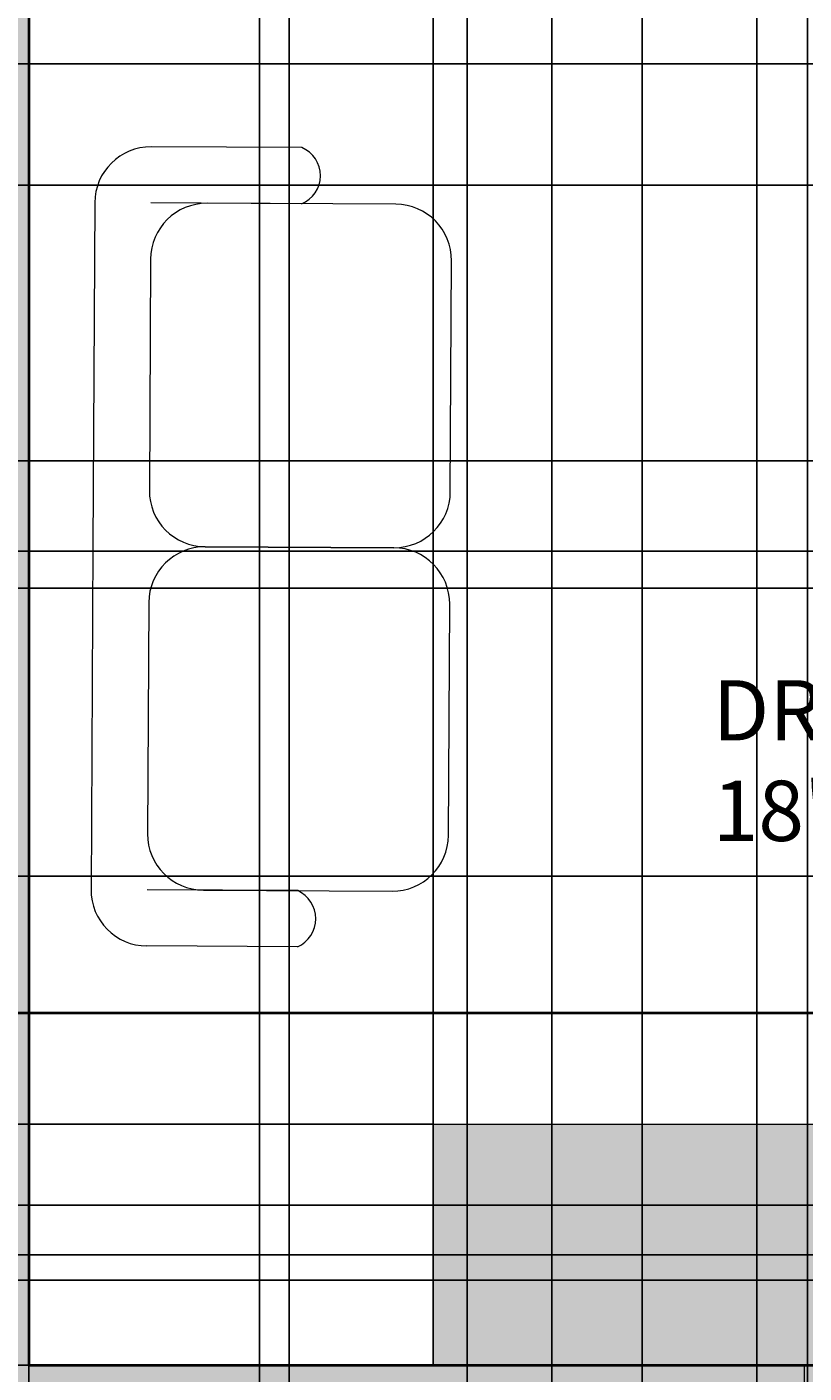
# Model space of a CAD drawing. Units: inches. Extents: x 818 to 1898, y 976 to 2364.
# Tile 23 of 96: x 1207 to 1284, y 1509 to 1643. Entities that reach past the tile are written whole.
import ezdxf

# ---------------------------------------------------------------- set-up
doc = ezdxf.new("R2010")
doc.units = ezdxf.units.IN
doc.header["$LTSCALE"] = 5
doc.header["$MEASUREMENT"] = 0
for name, color, linetype, lineweight in [('A-ANNO-DIMS', 2, 'Continuous', 18), ('A-AREA-IDEN', 7, 'Continuous', 18), ('A-FLOR-CASE', 8, 'Continuous', 18), ('A-FLOR-CASE-PATT', 33, 'Continuous', 9), ('A-FURN', 8, 'Continuous', 18), ('A-GLAZ', 4, 'Continuous', 18), ('A-WALL', 7, 'Continuous', 40)]:
    doc.layers.add(name, color=color, linetype=linetype, lineweight=lineweight)
doc.layers.add('A-GLAZ-PATT', color=141, linetype='Continuous', lineweight=9, true_color=0xadddf7)
doc.layers.add('A-WALL-PATT', color=251, linetype='Continuous', lineweight=13, true_color=0x636466)
doc.styles.get("Standard").update_dxf_attribs({"font": 'arial.ttf'})
doc.dimstyles.get("Standard").update_dxf_attribs({"dimtxt": 0.18, "dimasz": 0.18, "dimexe": 0.18, "dimexo": 0.0625, "dimgap": 0.09, "dimtad": 0, "dimtih": 1, "dimtoh": 1, "dimdec": 4, "dimzin": 0, "dimdsep": 46, "dimtxsty": 'Standard', "dimcen": 0.09, "dimadec": 0, "dimazin": 0, "dimtfac": 1, "dimtdec": 4, "dimtofl": 0, "dimtmove": 0, "dimatfit": 3, "dimfxl": 1, "dimtolj": 1, "dimtzin": 0, "dimarcsym": 0})

# ---------------------------------------------------------------- blocks, each defined once
blk = doc.blocks.new('*D59')
at = {"layer": 'A-ANNO-DIMS', "color": 0, "lineweight": -2, "ltscale": 5, "transparency": 16777216}
for p, q in [((1251.64, 2300.39), (818.03, 2300.39)), ((818.21, 2300.21), (818.21, 1669.95)), ((818.21, 1039.32), (818.21, 1669.59)), ((896.05, 1039.14), (818.03, 1039.14))]:
    blk.add_line(p, q, dxfattribs=at)
at = {"layer": 'A-ANNO-DIMS', "color": 0, "ltscale": 5, "transparency": 16777216}
for points in [[(818.18, 2300.21), (818.24, 2300.21), (818.21, 2300.39)], [(818.18, 1039.32), (818.24, 1039.32), (818.21, 1039.14)]]:
    blk.add_solid(points, dxfattribs=at)
at = {"layer": 'Defpoints', "color": 0, "ltscale": 5, "transparency": 16777216}
for p in [(818.21, 2300.39), (1251.71, 2300.39), (896.11, 1039.14)]:
    blk.add_point(p, dxfattribs=at)
at = {"layer": 'A-ANNO-DIMS', "color": 0, "ltscale": 5, "transparency": 16777216, "insert": (818.21, 1669.77), "char_height": 0.18, "attachment_point": 5}
blk.add_mtext('\\A1;1261.2', dxfattribs=at)
blk = doc.blocks.new('*D61')
at = {"layer": 'A-ANNO-DIMS', "color": 0, "lineweight": -2, "ltscale": 5, "transparency": 16777216}
for p, q in [((1071.73, 1203.03), (1071.73, 2363.87)), ((1071.91, 2363.69), (1250.94, 2363.69)), ((1430.55, 2363.69), (1251.51, 2363.69)), ((1430.73, 1203.03), (1430.73, 2363.87))]:
    blk.add_line(p, q, dxfattribs=at)
at = {"layer": 'A-ANNO-DIMS', "color": 0, "ltscale": 5, "transparency": 16777216}
for points in [[(1071.91, 2363.72), (1071.91, 2363.66), (1071.73, 2363.69)], [(1430.55, 2363.72), (1430.55, 2363.66), (1430.73, 2363.69)]]:
    blk.add_solid(points, dxfattribs=at)
at = {"layer": 'Defpoints', "color": 0, "ltscale": 5, "transparency": 16777216}
for p in [(1430.73, 2363.69), (1071.73, 1202.96), (1430.73, 1202.96)]:
    blk.add_point(p, dxfattribs=at)
at = {"layer": 'A-ANNO-DIMS', "color": 0, "ltscale": 5, "transparency": 16777216, "insert": (1251.23, 2363.69), "char_height": 0.18, "attachment_point": 5}
blk.add_mtext('\\A1;359', dxfattribs=at)
blk = doc.blocks.new('*D64')
at = {"layer": 'A-ANNO-DIMS', "color": 0, "lineweight": -2, "ltscale": 5, "transparency": 16777216}
for p, q in [((1197.73, 1501.14), (1197.73, 2363.87)), ((1197.91, 2363.69), (1313.93, 2363.69)), ((1430.55, 2363.69), (1314.52, 2363.69)), ((1430.73, 1501.14), (1430.73, 2363.87))]:
    blk.add_line(p, q, dxfattribs=at)
at = {"layer": 'A-ANNO-DIMS', "color": 0, "ltscale": 5, "transparency": 16777216}
for points in [[(1197.91, 2363.72), (1197.91, 2363.66), (1197.73, 2363.69)], [(1430.55, 2363.72), (1430.55, 2363.66), (1430.73, 2363.69)]]:
    blk.add_solid(points, dxfattribs=at)
at = {"layer": 'Defpoints', "color": 0, "ltscale": 5, "transparency": 16777216}
for p in [(1430.73, 2363.69), (1197.73, 1501.08), (1430.73, 1501.08)]:
    blk.add_point(p, dxfattribs=at)
at = {"layer": 'A-ANNO-DIMS', "color": 0, "ltscale": 5, "transparency": 16777216, "insert": (1314.23, 2363.69), "char_height": 0.18, "attachment_point": 5}
blk.add_mtext('\\A1;233', dxfattribs=at)
blk = doc.blocks.new('*D95')
at = {"layer": 'A-ANNO-DIMS', "color": 0, "lineweight": -2, "ltscale": 5, "transparency": 16777216}
for p, q in [((1173.54, 1071.12), (1173.54, 2363.87)), ((1173.72, 2363.69), (1201.29, 2363.69)), ((1229.47, 2363.69), (1201.9, 2363.69)), ((1229.65, 1071.12), (1229.65, 2363.87))]:
    blk.add_line(p, q, dxfattribs=at)
at = {"layer": 'A-ANNO-DIMS', "color": 0, "ltscale": 5, "transparency": 16777216}
for points in [[(1173.72, 2363.72), (1173.72, 2363.66), (1173.54, 2363.69)], [(1229.47, 2363.72), (1229.47, 2363.66), (1229.65, 2363.69)]]:
    blk.add_solid(points, dxfattribs=at)
at = {"layer": 'Defpoints', "color": 0, "ltscale": 5, "transparency": 16777216}
for p in [(1229.65, 2363.69), (1173.54, 1071.06), (1229.65, 1071.06)]:
    blk.add_point(p, dxfattribs=at)
at = {"layer": 'A-ANNO-DIMS', "color": 0, "ltscale": 5, "transparency": 16777216, "insert": (1201.59, 2363.69), "char_height": 0.18, "attachment_point": 5}
blk.add_mtext('\\A1;56.1', dxfattribs=at)
blk = doc.blocks.new('*D96')
at = {"layer": 'A-ANNO-DIMS', "color": 0, "lineweight": -2, "ltscale": 5, "transparency": 16777216}
for p, q in [((1229.65, 1071.12), (1229.65, 2363.87)), ((1229.83, 2363.69), (1256.52, 2363.69)), ((1283.99, 2363.69), (1257.3, 2363.69)), ((1284.17, 1071.12), (1284.17, 2363.87))]:
    blk.add_line(p, q, dxfattribs=at)
at = {"layer": 'A-ANNO-DIMS', "color": 0, "ltscale": 5, "transparency": 16777216}
for points in [[(1229.83, 2363.72), (1229.83, 2363.66), (1229.65, 2363.69)], [(1283.99, 2363.72), (1283.99, 2363.66), (1284.17, 2363.69)]]:
    blk.add_solid(points, dxfattribs=at)
at = {"layer": 'Defpoints', "color": 0, "ltscale": 5, "transparency": 16777216}
for p in [(1284.17, 2363.69), (1229.65, 1071.06), (1284.17, 1071.06)]:
    blk.add_point(p, dxfattribs=at)
at = {"layer": 'A-ANNO-DIMS', "color": 0, "ltscale": 5, "transparency": 16777216, "insert": (1256.91, 2363.69), "char_height": 0.18, "attachment_point": 5}
blk.add_mtext('\\A1;54.52', dxfattribs=at)
blk = doc.blocks.new('*D117')
at = {"layer": 'A-ANNO-DIMS', "color": 0, "lineweight": -2, "ltscale": 5, "transparency": 16777216}
for p, q in [((1766.29, 1545.18), (818.03, 1545.18)), ((818.21, 1545), (818.21, 1501.18)), ((818.21, 1456.99), (818.21, 1500.81)), ((1766.29, 1456.81), (818.03, 1456.81))]:
    blk.add_line(p, q, dxfattribs=at)
at = {"layer": 'A-ANNO-DIMS', "color": 0, "ltscale": 5, "transparency": 16777216}
for points in [[(818.18, 1545), (818.24, 1545), (818.21, 1545.18)], [(818.18, 1456.99), (818.24, 1456.99), (818.21, 1456.81)]]:
    blk.add_solid(points, dxfattribs=at)
at = {"layer": 'Defpoints', "color": 0, "ltscale": 5, "transparency": 16777216}
for p in [(818.21, 1545.18), (1766.35, 1545.18), (1766.35, 1456.81)]:
    blk.add_point(p, dxfattribs=at)
at = {"layer": 'A-ANNO-DIMS', "color": 0, "ltscale": 5, "transparency": 16777216, "insert": (818.21, 1501), "char_height": 0.18, "attachment_point": 5}
blk.add_mtext('\\A1;88.37', dxfattribs=at)
blk = doc.blocks.new('*D118')
at = {"layer": 'A-ANNO-DIMS', "color": 0, "lineweight": -2, "ltscale": 5, "transparency": 16777216}
for p, q in [((1766.29, 1627.51), (818.03, 1627.51)), ((818.21, 1627.33), (818.21, 1586.53)), ((818.21, 1545.36), (818.21, 1586.16)), ((1766.29, 1545.18), (818.03, 1545.18))]:
    blk.add_line(p, q, dxfattribs=at)
at = {"layer": 'A-ANNO-DIMS', "color": 0, "ltscale": 5, "transparency": 16777216}
for points in [[(818.18, 1627.33), (818.24, 1627.33), (818.21, 1627.51)], [(818.18, 1545.36), (818.24, 1545.36), (818.21, 1545.18)]]:
    blk.add_solid(points, dxfattribs=at)
at = {"layer": 'Defpoints', "color": 0, "ltscale": 5, "transparency": 16777216}
for p in [(818.21, 1627.51), (1766.35, 1627.51), (1766.35, 1545.18)]:
    blk.add_point(p, dxfattribs=at)
at = {"layer": 'A-ANNO-DIMS', "color": 0, "ltscale": 5, "transparency": 16777216, "insert": (818.21, 1586.34), "char_height": 0.18, "attachment_point": 5}
blk.add_mtext('\\A1;82.32', dxfattribs=at)
blk = doc.blocks.new('*D119')
at = {"layer": 'A-ANNO-DIMS', "color": 0, "lineweight": -2, "ltscale": 5, "transparency": 16777216}
for p, q in [((1766.29, 1716.99), (818.03, 1716.99)), ((818.21, 1716.81), (818.21, 1672.43)), ((818.21, 1627.69), (818.21, 1672.06)), ((1766.29, 1627.51), (818.03, 1627.51))]:
    blk.add_line(p, q, dxfattribs=at)
at = {"layer": 'A-ANNO-DIMS', "color": 0, "ltscale": 5, "transparency": 16777216}
for points in [[(818.18, 1716.81), (818.24, 1716.81), (818.21, 1716.99)], [(818.18, 1627.69), (818.24, 1627.69), (818.21, 1627.51)]]:
    blk.add_solid(points, dxfattribs=at)
at = {"layer": 'Defpoints', "color": 0, "ltscale": 5, "transparency": 16777216}
for p in [(818.21, 1716.99), (1766.35, 1716.99), (1766.35, 1627.51)]:
    blk.add_point(p, dxfattribs=at)
at = {"layer": 'A-ANNO-DIMS', "color": 0, "ltscale": 5, "transparency": 16777216, "insert": (818.21, 1672.25), "char_height": 0.18, "attachment_point": 5}
blk.add_mtext('\\A1;89.48', dxfattribs=at)
blk = doc.blocks.new('*D145')
at = {"layer": 'A-ANNO-DIMS', "color": 0, "lineweight": -2, "ltscale": 5, "transparency": 16777216}
for p, q in [((1197.39, 2122.31), (1197.39, 975.66)), ((1232.61, 2122.31), (1232.61, 975.66)), ((1197.57, 975.84), (1214.61, 975.84)), ((1232.43, 975.84), (1215.39, 975.84))]:
    blk.add_line(p, q, dxfattribs=at)
at = {"layer": 'A-ANNO-DIMS', "color": 0, "ltscale": 5, "transparency": 16777216}
for points in [[(1197.57, 975.87), (1197.57, 975.81), (1197.39, 975.84)], [(1232.43, 975.87), (1232.43, 975.81), (1232.61, 975.84)]]:
    blk.add_solid(points, dxfattribs=at)
at = {"layer": 'Defpoints', "color": 0, "ltscale": 5, "transparency": 16777216}
for p in [(1197.39, 2122.38), (1232.61, 2122.38), (1232.61, 975.84)]:
    blk.add_point(p, dxfattribs=at)
at = {"layer": 'A-ANNO-DIMS', "color": 0, "ltscale": 5, "transparency": 16777216, "insert": (1215, 975.84), "char_height": 0.18, "attachment_point": 5}
blk.add_mtext('\\A1;35.22', dxfattribs=at)
blk = doc.blocks.new('*D159')
at = {"layer": 'A-ANNO-DIMS', "color": 0, "lineweight": -2, "ltscale": 5, "transparency": 16777216}
for p, q in [((1206.73, 1687.02), (1206.73, 975.66)), ((1463.73, 1687.02), (1463.73, 975.66)), ((1206.91, 975.84), (1334.93, 975.84)), ((1463.55, 975.84), (1335.52, 975.84))]:
    blk.add_line(p, q, dxfattribs=at)
at = {"layer": 'A-ANNO-DIMS', "color": 0, "ltscale": 5, "transparency": 16777216}
for points in [[(1206.91, 975.87), (1206.91, 975.81), (1206.73, 975.84)], [(1463.55, 975.87), (1463.55, 975.81), (1463.73, 975.84)]]:
    blk.add_solid(points, dxfattribs=at)
at = {"layer": 'Defpoints', "color": 0, "ltscale": 5, "transparency": 16777216}
for p in [(1206.73, 1687.08), (1463.73, 1687.08), (1463.73, 975.84)]:
    blk.add_point(p, dxfattribs=at)
at = {"layer": 'A-ANNO-DIMS', "color": 0, "ltscale": 5, "transparency": 16777216, "insert": (1335.23, 975.84), "char_height": 0.18, "attachment_point": 5}
blk.add_mtext('\\A1;257', dxfattribs=at)
blk = doc.blocks.new('*D181')
at = {"layer": 'A-ANNO-DIMS', "color": 0, "lineweight": -2, "ltscale": 5, "transparency": 16777216}
for p, q in [((1599.66, 1639.58), (818.03, 1639.58)), ((818.21, 1639.4), (818.21, 1620.01)), ((818.21, 1600.26), (818.21, 1619.65)), ((1619.66, 1600.08), (818.03, 1600.08))]:
    blk.add_line(p, q, dxfattribs=at)
at = {"layer": 'A-ANNO-DIMS', "color": 0, "ltscale": 5, "transparency": 16777216}
for points in [[(818.18, 1639.4), (818.24, 1639.4), (818.21, 1639.58)], [(818.18, 1600.26), (818.24, 1600.26), (818.21, 1600.08)]]:
    blk.add_solid(points, dxfattribs=at)
at = {"layer": 'Defpoints', "color": 0, "ltscale": 5, "transparency": 16777216}
for p in [(1599.73, 1639.58), (818.21, 1600.08), (1619.73, 1600.08)]:
    blk.add_point(p, dxfattribs=at)
at = {"layer": 'A-ANNO-DIMS', "color": 0, "ltscale": 5, "transparency": 16777216, "insert": (818.21, 1619.83), "char_height": 0.18, "attachment_point": 5}
blk.add_mtext('\\A1;39.5', dxfattribs=at)
blk = doc.blocks.new('*D187')
at = {"layer": 'A-ANNO-DIMS', "color": 0, "lineweight": -2, "ltscale": 5, "transparency": 16777216}
for p, q in [((1705.66, 1545.08), (818.03, 1545.08)), ((818.21, 1544.9), (818.21, 1533.26)), ((818.21, 1521.26), (818.21, 1532.9)), ((1705.66, 1521.08), (818.03, 1521.08))]:
    blk.add_line(p, q, dxfattribs=at)
at = {"layer": 'A-ANNO-DIMS', "color": 0, "ltscale": 5, "transparency": 16777216}
for points in [[(818.18, 1544.9), (818.24, 1544.9), (818.21, 1545.08)], [(818.18, 1521.26), (818.24, 1521.26), (818.21, 1521.08)]]:
    blk.add_solid(points, dxfattribs=at)
at = {"layer": 'Defpoints', "color": 0, "ltscale": 5, "transparency": 16777216}
for p in [(818.21, 1545.08), (1705.73, 1545.08), (1705.73, 1521.08)]:
    blk.add_point(p, dxfattribs=at)
at = {"layer": 'A-ANNO-DIMS', "color": 0, "ltscale": 5, "transparency": 16777216, "insert": (818.21, 1533.08), "char_height": 0.18, "attachment_point": 5}
blk.add_mtext('\\A1;24', dxfattribs=at)
blk = doc.blocks.new('*D194')
at = {"layer": 'A-ANNO-DIMS', "color": 0, "lineweight": -2, "ltscale": 5, "transparency": 16777216}
for p, q in [((1616.66, 1591.08), (818.03, 1591.08)), ((818.21, 1590.9), (818.21, 1575.1)), ((818.21, 1558.93), (818.21, 1574.73)), ((1616.66, 1558.75), (818.03, 1558.75))]:
    blk.add_line(p, q, dxfattribs=at)
at = {"layer": 'A-ANNO-DIMS', "color": 0, "ltscale": 5, "transparency": 16777216}
for points in [[(818.18, 1590.9), (818.24, 1590.9), (818.21, 1591.08)], [(818.18, 1558.93), (818.24, 1558.93), (818.21, 1558.75)]]:
    blk.add_solid(points, dxfattribs=at)
at = {"layer": 'Defpoints', "color": 0, "ltscale": 5, "transparency": 16777216}
for p in [(818.21, 1591.08), (1616.73, 1591.08), (1616.73, 1558.75)]:
    blk.add_point(p, dxfattribs=at)
at = {"layer": 'A-ANNO-DIMS', "color": 0, "ltscale": 5, "transparency": 16777216, "insert": (818.21, 1574.92), "char_height": 0.18, "attachment_point": 5}
blk.add_mtext('\\A1;32.326', dxfattribs=at)
blk = doc.blocks.new('*D201')
at = {"layer": 'A-ANNO-DIMS', "color": 0, "lineweight": -2, "ltscale": 5, "transparency": 16777216}
for p, q in [((1678.27, 1518.56), (818.03, 1518.56)), ((818.21, 1518.38), (818.21, 1498.18)), ((818.21, 1477.61), (818.21, 1497.81)), ((1678.27, 1477.43), (818.03, 1477.43))]:
    blk.add_line(p, q, dxfattribs=at)
at = {"layer": 'A-ANNO-DIMS', "color": 0, "ltscale": 5, "transparency": 16777216}
for points in [[(818.18, 1518.38), (818.24, 1518.38), (818.21, 1518.56)], [(818.18, 1477.61), (818.24, 1477.61), (818.21, 1477.43)]]:
    blk.add_solid(points, dxfattribs=at)
at = {"layer": 'Defpoints', "color": 0, "ltscale": 5, "transparency": 16777216}
for p in [(818.21, 1518.56), (1678.33, 1518.56), (1678.33, 1477.43)]:
    blk.add_point(p, dxfattribs=at)
at = {"layer": 'A-ANNO-DIMS', "color": 0, "ltscale": 5, "transparency": 16777216, "insert": (818.21, 1497.99), "char_height": 0.18, "attachment_point": 5}
blk.add_mtext('\\A1;41.135', dxfattribs=at)
blk = doc.blocks.new('*D233')
at = {"layer": 'A-ANNO-DIMS', "color": 0, "lineweight": -2, "ltscale": 5, "transparency": 16777216}
for p, q in [((1267.73, 2044.02), (1267.73, 975.66)), ((1303.93, 2008.33), (1303.93, 975.66)), ((1267.91, 975.84), (1285.36, 975.84)), ((1303.75, 975.84), (1286.29, 975.84))]:
    blk.add_line(p, q, dxfattribs=at)
at = {"layer": 'A-ANNO-DIMS', "color": 0, "ltscale": 5, "transparency": 16777216}
for points in [[(1267.91, 975.87), (1267.91, 975.81), (1267.73, 975.84)], [(1303.75, 975.87), (1303.75, 975.81), (1303.93, 975.84)]]:
    blk.add_solid(points, dxfattribs=at)
at = {"layer": 'Defpoints', "color": 0, "ltscale": 5, "transparency": 16777216}
for p in [(1267.73, 2044.08), (1303.93, 2008.39), (1303.93, 975.84)]:
    blk.add_point(p, dxfattribs=at)
at = {"layer": 'A-ANNO-DIMS', "color": 0, "ltscale": 5, "transparency": 16777216, "insert": (1285.83, 975.84), "char_height": 0.18, "attachment_point": 5}
blk.add_mtext('\\A1;36.206', dxfattribs=at)
blk = doc.blocks.new('*D251')
at = {"layer": 'A-ANNO-DIMS', "color": 0, "lineweight": -2, "ltscale": 5, "transparency": 16777216}
for p, q in [((1250.3, 1878.33), (1250.3, 975.66)), ((1258.73, 1878.33), (1258.73, 975.66)), ((1250.48, 975.84), (1254.12, 975.84)), ((1258.55, 975.84), (1254.91, 975.84))]:
    blk.add_line(p, q, dxfattribs=at)
at = {"layer": 'A-ANNO-DIMS', "color": 0, "ltscale": 5, "transparency": 16777216}
for points in [[(1250.48, 975.87), (1250.48, 975.81), (1250.3, 975.84)], [(1258.55, 975.87), (1258.55, 975.81), (1258.73, 975.84)]]:
    blk.add_solid(points, dxfattribs=at)
at = {"layer": 'Defpoints', "color": 0, "ltscale": 5, "transparency": 16777216}
for p in [(1250.3, 1878.39), (1258.73, 1878.39), (1258.73, 975.84)]:
    blk.add_point(p, dxfattribs=at)
at = {"layer": 'A-ANNO-DIMS', "color": 0, "ltscale": 5, "transparency": 16777216, "insert": (1254.51, 975.84), "char_height": 0.18, "attachment_point": 5}
blk.add_mtext('\\A1;8.422', dxfattribs=at)
blk = doc.blocks.new('*D254')
at = {"layer": 'A-ANNO-DIMS', "color": 0, "lineweight": -2, "ltscale": 5, "transparency": 16777216}
for p, q in [((1267.73, 2044.02), (1267.73, 975.66)), ((1330.3, 2044.02), (1330.3, 975.66)), ((1267.91, 975.84), (1298.62, 975.84)), ((1330.12, 975.84), (1299.41, 975.84))]:
    blk.add_line(p, q, dxfattribs=at)
at = {"layer": 'A-ANNO-DIMS', "color": 0, "ltscale": 5, "transparency": 16777216}
for points in [[(1267.91, 975.87), (1267.91, 975.81), (1267.73, 975.84)], [(1330.12, 975.87), (1330.12, 975.81), (1330.3, 975.84)]]:
    blk.add_solid(points, dxfattribs=at)
at = {"layer": 'Defpoints', "color": 0, "ltscale": 5, "transparency": 16777216}
for p in [(1267.73, 2044.08), (1330.3, 2044.08), (1330.3, 975.84)]:
    blk.add_point(p, dxfattribs=at)
at = {"layer": 'A-ANNO-DIMS', "color": 0, "ltscale": 5, "transparency": 16777216, "insert": (1299.02, 975.84), "char_height": 0.18, "attachment_point": 5}
blk.add_mtext('\\A1;62.58', dxfattribs=at)
blk = doc.blocks.new('*D269')
at = {"layer": 'A-ANNO-DIMS', "color": 0, "lineweight": -2, "ltscale": 5, "transparency": 16777216}
for p, q in [((1246.94, 1534.14), (1246.94, 2363.87)), ((1247.12, 2363.69), (1293.71, 2363.69)), ((1341.08, 2363.69), (1294.49, 2363.69)), ((1341.26, 1534.14), (1341.26, 2363.87))]:
    blk.add_line(p, q, dxfattribs=at)
at = {"layer": 'A-ANNO-DIMS', "color": 0, "ltscale": 5, "transparency": 16777216}
for points in [[(1247.12, 2363.72), (1247.12, 2363.66), (1246.94, 2363.69)], [(1341.08, 2363.72), (1341.08, 2363.66), (1341.26, 2363.69)]]:
    blk.add_solid(points, dxfattribs=at)
at = {"layer": 'Defpoints', "color": 0, "ltscale": 5, "transparency": 16777216}
for p in [(1341.26, 2363.69), (1246.94, 1534.08), (1341.26, 1534.08)]:
    blk.add_point(p, dxfattribs=at)
at = {"layer": 'A-ANNO-DIMS', "color": 0, "ltscale": 5, "transparency": 16777216, "insert": (1294.1, 2363.69), "char_height": 0.18, "attachment_point": 5}
blk.add_mtext('\\A1;94.32', dxfattribs=at)
blk = doc.blocks.new('*D270')
at = {"layer": 'A-ANNO-DIMS', "color": 0, "lineweight": -2, "ltscale": 5, "transparency": 16777216}
for p, q in [((1246.88, 1534.08), (818.03, 1534.08)), ((818.21, 1533.9), (818.21, 1522.26)), ((818.21, 1510.26), (818.21, 1521.9)), ((1246.88, 1510.08), (818.03, 1510.08))]:
    blk.add_line(p, q, dxfattribs=at)
at = {"layer": 'A-ANNO-DIMS', "color": 0, "ltscale": 5, "transparency": 16777216}
for points in [[(818.18, 1533.9), (818.24, 1533.9), (818.21, 1534.08)], [(818.18, 1510.26), (818.24, 1510.26), (818.21, 1510.08)]]:
    blk.add_solid(points, dxfattribs=at)
at = {"layer": 'Defpoints', "color": 0, "ltscale": 5, "transparency": 16777216}
for p in [(818.21, 1534.08), (1246.94, 1534.08), (1246.94, 1510.08)]:
    blk.add_point(p, dxfattribs=at)
at = {"layer": 'A-ANNO-DIMS', "color": 0, "ltscale": 5, "transparency": 16777216, "insert": (818.21, 1522.08), "char_height": 0.18, "attachment_point": 5}
blk.add_mtext('\\A1;24', dxfattribs=at)
blk = doc.blocks.new('*D271')
at = {"layer": 'A-ANNO-DIMS', "color": 0, "lineweight": -2, "ltscale": 5, "transparency": 16777216}
for p, q in [((1206.73, 1510.14), (1206.73, 2363.87)), ((1206.91, 2363.69), (1226.45, 2363.69)), ((1246.76, 2363.69), (1227.21, 2363.69)), ((1246.94, 1510.14), (1246.94, 2363.87))]:
    blk.add_line(p, q, dxfattribs=at)
at = {"layer": 'A-ANNO-DIMS', "color": 0, "ltscale": 5, "transparency": 16777216}
for points in [[(1206.91, 2363.72), (1206.91, 2363.66), (1206.73, 2363.69)], [(1246.76, 2363.72), (1246.76, 2363.66), (1246.94, 2363.69)]]:
    blk.add_solid(points, dxfattribs=at)
at = {"layer": 'Defpoints', "color": 0, "ltscale": 5, "transparency": 16777216}
for p in [(1246.94, 2363.69), (1206.73, 1510.08), (1246.94, 1510.08)]:
    blk.add_point(p, dxfattribs=at)
at = {"layer": 'A-ANNO-DIMS', "color": 0, "ltscale": 5, "transparency": 16777216, "insert": (1226.83, 2363.69), "char_height": 0.18, "attachment_point": 5}
blk.add_mtext('\\A1;40.21', dxfattribs=at)
blk = doc.blocks.new('*D272')
at = {"layer": 'A-ANNO-DIMS', "color": 0, "lineweight": -2, "ltscale": 5, "transparency": 16777216}
for p, q in [((1406.66, 1587.42), (818.03, 1587.42)), ((818.21, 1587.24), (818.21, 1556.89)), ((818.21, 1526.18), (818.21, 1556.52)), ((1406.66, 1526), (818.03, 1526))]:
    blk.add_line(p, q, dxfattribs=at)
at = {"layer": 'A-ANNO-DIMS', "color": 0, "ltscale": 5, "transparency": 16777216}
for points in [[(818.18, 1587.24), (818.24, 1587.24), (818.21, 1587.42)], [(818.18, 1526.18), (818.24, 1526.18), (818.21, 1526)]]:
    blk.add_solid(points, dxfattribs=at)
at = {"layer": 'Defpoints', "color": 0, "ltscale": 5, "transparency": 16777216}
for p in [(818.21, 1587.42), (1406.73, 1587.42), (1406.73, 1526)]:
    blk.add_point(p, dxfattribs=at)
at = {"layer": 'A-ANNO-DIMS', "color": 0, "ltscale": 5, "transparency": 16777216, "insert": (818.21, 1556.71), "char_height": 0.18, "attachment_point": 5}
blk.add_mtext('\\A1;61.42', dxfattribs=at)
blk = doc.blocks.new('*D278')
at = {"layer": 'A-ANNO-DIMS', "color": 0, "lineweight": -2, "ltscale": 5, "transparency": 16777216}
for p, q in [((1324.03, 1700.74), (1324.03, 975.66)), ((1267.73, 1696.02), (1267.73, 975.66)), ((1267.91, 975.84), (1295.5, 975.84)), ((1323.85, 975.84), (1296.26, 975.84))]:
    blk.add_line(p, q, dxfattribs=at)
at = {"layer": 'A-ANNO-DIMS', "color": 0, "ltscale": 5, "transparency": 16777216}
for points in [[(1267.91, 975.87), (1267.91, 975.81), (1267.73, 975.84)], [(1323.85, 975.87), (1323.85, 975.81), (1324.03, 975.84)]]:
    blk.add_solid(points, dxfattribs=at)
at = {"layer": 'Defpoints', "color": 0, "ltscale": 5, "transparency": 16777216}
for p in [(1324.03, 1700.81), (1267.73, 1696.08), (1324.03, 975.84)]:
    blk.add_point(p, dxfattribs=at)
at = {"layer": 'A-ANNO-DIMS', "color": 0, "ltscale": 5, "transparency": 16777216, "insert": (1295.88, 975.84), "char_height": 0.18, "attachment_point": 5}
blk.add_mtext('\\A1;56.31', dxfattribs=at)
blk = doc.blocks.new('*D279')
at = {"layer": 'A-ANNO-DIMS', "color": 0, "lineweight": -2, "ltscale": 5, "transparency": 16777216}
for p, q in [((1279.13, 1713.75), (1279.13, 975.66)), ((1267.73, 1696.02), (1267.73, 975.66)), ((1267.91, 975.84), (1273.11, 975.84)), ((1278.95, 975.84), (1273.74, 975.84))]:
    blk.add_line(p, q, dxfattribs=at)
at = {"layer": 'A-ANNO-DIMS', "color": 0, "ltscale": 5, "transparency": 16777216}
for points in [[(1267.91, 975.87), (1267.91, 975.81), (1267.73, 975.84)], [(1278.95, 975.87), (1278.95, 975.81), (1279.13, 975.84)]]:
    blk.add_solid(points, dxfattribs=at)
at = {"layer": 'Defpoints', "color": 0, "ltscale": 5, "transparency": 16777216}
for p in [(1279.13, 1713.82), (1267.73, 1696.08), (1267.73, 975.84)]:
    blk.add_point(p, dxfattribs=at)
at = {"layer": 'A-ANNO-DIMS', "color": 0, "ltscale": 5, "transparency": 16777216, "insert": (1273.43, 975.84), "char_height": 0.18, "attachment_point": 5}
blk.add_mtext('\\A1;11.4', dxfattribs=at)
blk = doc.blocks.new('*D283')
at = {"layer": 'A-ANNO-DIMS', "color": 0, "lineweight": -2, "ltscale": 5, "transparency": 16777216}
for p, q in [((1351.6, 1761.39), (1351.6, 975.66)), ((1267.73, 1696.02), (1267.73, 975.66)), ((1267.91, 975.84), (1309.27, 975.84)), ((1351.42, 975.84), (1310.06, 975.84))]:
    blk.add_line(p, q, dxfattribs=at)
at = {"layer": 'A-ANNO-DIMS', "color": 0, "ltscale": 5, "transparency": 16777216}
for points in [[(1267.91, 975.87), (1267.91, 975.81), (1267.73, 975.84)], [(1351.42, 975.87), (1351.42, 975.81), (1351.6, 975.84)]]:
    blk.add_solid(points, dxfattribs=at)
at = {"layer": 'Defpoints', "color": 0, "ltscale": 5, "transparency": 16777216}
for p in [(1351.6, 1761.45), (1267.73, 1696.08), (1351.6, 975.84)]:
    blk.add_point(p, dxfattribs=at)
at = {"layer": 'A-ANNO-DIMS', "color": 0, "ltscale": 5, "transparency": 16777216, "insert": (1309.66, 975.84), "char_height": 0.18, "attachment_point": 5}
blk.add_mtext('\\A1;83.87', dxfattribs=at)
blk = doc.blocks.new('*D285')
at = {"layer": 'A-ANNO-DIMS', "color": 0, "lineweight": -2, "ltscale": 5, "transparency": 16777216}
for p, q in [((1305.83, 1830.02), (1305.83, 975.66)), ((1267.73, 1814.9), (1267.73, 975.66)), ((1267.91, 975.84), (1286.47, 975.84)), ((1305.65, 975.84), (1287.08, 975.84))]:
    blk.add_line(p, q, dxfattribs=at)
at = {"layer": 'A-ANNO-DIMS', "color": 0, "ltscale": 5, "transparency": 16777216}
for points in [[(1267.91, 975.87), (1267.91, 975.81), (1267.73, 975.84)], [(1305.65, 975.87), (1305.65, 975.81), (1305.83, 975.84)]]:
    blk.add_solid(points, dxfattribs=at)
at = {"layer": 'Defpoints', "color": 0, "ltscale": 5, "transparency": 16777216}
for p in [(1305.83, 1830.08), (1267.73, 1814.97), (1267.73, 975.84)]:
    blk.add_point(p, dxfattribs=at)
at = {"layer": 'A-ANNO-DIMS', "color": 0, "ltscale": 5, "transparency": 16777216, "insert": (1286.78, 975.84), "char_height": 0.18, "attachment_point": 5}
blk.add_mtext('\\A1;38.1', dxfattribs=at)
blk = doc.blocks.new('*D291')
at = {"layer": 'A-ANNO-DIMS', "color": 0, "lineweight": -2, "ltscale": 5, "transparency": 16777216}
for p, q in [((1206.79, 1687.08), (1897.92, 1687.08)), ((1897.74, 1686.9), (1897.74, 1647.61)), ((1897.74, 1607.95), (1897.74, 1647.24)), ((1318.96, 1607.77), (1897.92, 1607.77))]:
    blk.add_line(p, q, dxfattribs=at)
at = {"layer": 'A-ANNO-DIMS', "color": 0, "ltscale": 5, "transparency": 16777216}
for points in [[(1897.71, 1686.9), (1897.77, 1686.9), (1897.74, 1687.08)], [(1897.71, 1607.95), (1897.77, 1607.95), (1897.74, 1607.77)]]:
    blk.add_solid(points, dxfattribs=at)
at = {"layer": 'Defpoints', "color": 0, "ltscale": 5, "transparency": 16777216}
for p in [(1206.73, 1687.08), (1897.74, 1687.08), (1318.89, 1607.77)]:
    blk.add_point(p, dxfattribs=at)
at = {"layer": 'A-ANNO-DIMS', "color": 0, "ltscale": 5, "transparency": 16777216, "insert": (1897.74, 1647.42), "char_height": 0.18, "attachment_point": 5}
blk.add_mtext('\\A1;79.3', dxfattribs=at)

msp = doc.modelspace()

# ---------------------------------------------------------------- hatches: boundary and pattern name
at = {"layer": 'A-FLOR-CASE-PATT', "ltscale": 5}
h = msp.add_hatch(color=256, dxfattribs=at)
h.dxf.hatch_style = 1
h.paths.add_polyline_path([(1705.7251, 1941.0782), (1681.7252, 1941.0782), (1681.7252, 1900.0782), (1599.7251, 1900.0782), (1599.7251, 1876.0782), (1705.7251, 1876.0782)])
h.paths.add_polyline_path([(1457.7252, 1409.1177), (1457.7252, 1526.6712), (1439.7252, 1526.6712), (1439.7252, 1457.5313), (1446.3307, 1457.5313), (1446.3307, 1468.9514), (1446.8307, 1470.665), (1446.8307, 1469.665), (1446.8307, 1468.9514), (1446.8307, 1456.8361), (1446.8307, 1444.7258), (1446.8307, 1443.3338), (1446.3307, 1444.7258), (1446.3307, 1456.8361), (1439.7252, 1456.8361), (1439.7252, 1355.0782), (1463.7251, 1355.0782), (1463.7251, 1367.3287), (1458.0475, 1367.3287, -0.23606798), (1457.0475, 1369.3287), (1456.0475, 1369.3287, -0.11764706), (1456.0475, 1386.3287), (1457.0475, 1386.3287, -0.23606798), (1458.0475, 1388.3287), (1463.7251, 1388.3287), (1463.7251, 1389.3211)])
h.paths.add_polyline_path([(1341.2593, 1534.0782), (1246.9377, 1534.0782), (1246.9377, 1510.0782), (1341.2593, 1510.0782)])
h.paths.add_polyline_path([(1288.8272, 1519.927), (1289.8272, 1519.927), (1290.5408, 1519.927), (1302.6561, 1519.927), (1314.7664, 1519.927), (1316.1584, 1519.927), (1314.7664, 1519.427), (1302.6561, 1519.427), (1302.6561, 1512.8214), (1301.9609, 1512.8214), (1301.9609, 1519.427), (1290.5408, 1519.427)], flags=16)
h.paths.add_polyline_path([(1377.7791, 1867.0782), (1344.5531, 1867.0782), (1344.5531, 1860.4726), (1355.9731, 1860.4726), (1357.6867, 1859.9726), (1356.6867, 1859.9726), (1355.9731, 1859.9726), (1343.8579, 1859.9726), (1331.7475, 1859.9726), (1330.3556, 1859.9726), (1331.7475, 1860.4726), (1343.8579, 1860.4726), (1343.8579, 1867.0782), (1311.3271, 1867.0782), (1311.3271, 1853.7496), (1377.7791, 1853.7496)])
h.paths.add_polyline_path([(1301.148, 1610.7299, -0.46196039), (1314.4882, 1599.3725, -0.19222541), (1311.3254, 1591.4497, 0.54791519), (1336.8832, 1607.7707, 0.92061359)])
h.paths.add_polyline_path([(1370.719, 1780.5695, 1), (1332.478, 1780.5695, 1)])
h.paths.add_polyline_path([(1705.7251, 1463.0782), (1681.7252, 1463.0782), (1681.7252, 1379.0782), (1622.7252, 1379.0782), (1622.7252, 1355.0782), (1705.7251, 1355.0782)])
h.paths.add_polyline_path([(1658.1052, 1359.2188), (1658.1786, 1359.2188), (1658.1786, 1373.8763), (1658.1052, 1373.9202)], flags=16)
h.paths.add_polyline_path([(1686.9271, 1409.9311), (1686.8832, 1409.8578), (1701.5845, 1409.8578), (1701.5845, 1409.9311)], flags=16)
h.paths.add_polyline_path([(1637.1266, 1359.2188), (1637.2, 1359.2188), (1637.2, 1373.8763), (1637.1266, 1373.9202)], flags=16)
at = {"layer": 'A-GLAZ-PATT', "ltscale": 5}
h = msp.add_hatch(color=256, dxfattribs=at)
h.dxf.hatch_style = 1
h.paths.add_polyline_path([(1283.8183, 1504.5782), (1206.7251, 1504.5782), (1206.7251, 1501.0782), (1283.8183, 1501.0782)])
h.paths.add_polyline_path([(1283.8183, 1510.0782), (1206.7251, 1510.0782), (1206.7251, 1506.5782), (1283.8183, 1506.5782)])
h.paths.add_polyline_path([(1490.9163, 1355.0782), (1439.7252, 1355.0782), (1439.7252, 1409.0522), (1436.2252, 1409.0522), (1436.2252, 1351.5782), (1490.9163, 1351.5782)])
h.paths.add_polyline_path([(1434.2252, 1409.0522), (1430.7251, 1409.0522), (1430.7251, 1346.0782), (1435.0799, 1346.0782), (1435.0731, 1346.1152), (1435.1501, 1346.0782), (1490.9163, 1346.0782), (1490.9163, 1349.5782), (1434.2252, 1349.5782)])
h.paths.add_polyline_path([(1714.7252, 1545.0782), (1711.2252, 1545.0782), (1711.2252, 1521.0782), (1714.7252, 1521.0782)])
h.paths.add_polyline_path([(1709.2252, 1545.0782), (1705.7251, 1545.0782), (1705.7251, 1521.0782), (1709.2252, 1521.0782)])
h.paths.add_polyline_path([(1714.7252, 1687.0782), (1711.2252, 1687.0782), (1711.2252, 1649.9029), (1714.7252, 1649.9029)])
h.paths.add_polyline_path([(1709.2252, 1687.0782), (1705.7251, 1687.0782), (1705.7251, 1649.9029), (1709.2252, 1649.9029)])
h.paths.add_polyline_path([(1709.2252, 1745.5584), (1705.7251, 1745.5584), (1705.7251, 1717.3178), (1709.2252, 1717.3178)])
h.paths.add_polyline_path([(1714.7252, 1745.5584), (1711.2252, 1745.5584), (1711.2252, 1717.3178), (1714.7252, 1717.3178)])
h.paths.add_polyline_path([(1714.7252, 2014.5114), (1711.2252, 2014.5114), (1711.2252, 1962.0338), (1714.7252, 1962.0338)])
h.paths.add_polyline_path([(1709.2252, 2014.5114), (1705.7251, 2014.5114), (1705.7251, 1962.0338), (1709.2252, 1962.0338)])
h.paths.add_polyline_path([(1538.5155, 2047.5782), (1485.1216, 2047.5782), (1485.1216, 2044.0782), (1538.5155, 2044.0782)])
h.paths.add_polyline_path([(1538.5155, 2053.0782), (1485.1216, 2053.0782), (1485.1216, 2049.5782), (1538.5155, 2049.5782)])
h.paths.add_polyline_path([(1388.0315, 2047.5782), (1330.305, 2047.5782), (1330.305, 2044.0782), (1388.0315, 2044.0782)])
h.paths.add_polyline_path([(1388.0315, 2053.0782), (1330.305, 2053.0782), (1330.305, 2049.5782), (1388.0315, 2049.5782)])
h.paths.add_polyline_path([(1262.2252, 2019.2871), (1258.7251, 2019.2871), (1258.7251, 1928.9218), (1262.2252, 1928.9218)])
h.paths.add_polyline_path([(1267.7251, 2019.2871), (1264.2252, 2019.2871), (1264.2252, 1928.9218), (1267.7251, 1928.9218)])
h.paths.add_polyline_path([(1262.2252, 1862.9652), (1258.7251, 1862.9652), (1258.7251, 1814.9652), (1262.2252, 1814.9652)])
h.paths.add_polyline_path([(1267.7251, 1862.9652), (1264.2252, 1862.9652), (1264.2252, 1814.9652), (1267.7251, 1814.9652)])
h.paths.add_polyline_path([(1262.2252, 1755.3321), (1258.7251, 1755.3321), (1258.7251, 1707.3321), (1262.2252, 1707.3321)])
h.paths.add_polyline_path([(1267.7251, 1755.3321), (1264.2252, 1755.3321), (1264.2252, 1707.3321), (1267.7251, 1707.3321)])
h.paths.add_polyline_path([(1251.9333, 1692.5782), (1206.7251, 1692.5782), (1206.7251, 1687.0782), (1251.9333, 1687.0782)])
h.paths.add_polyline_path([(1251.9333, 1700.0782), (1206.7251, 1700.0782), (1206.7251, 1694.5782), (1251.9333, 1694.5782)])
at = {"layer": 'A-WALL-PATT', "ltscale": 5}
h = msp.add_hatch(color=256, dxfattribs=at)
h.dxf.hatch_style = 1
h.paths.add_polyline_path([(1206.7251, 1687.0782), (1206.7251, 1700.0782), (1197.7251, 1700.0782), (1197.7251, 1501.0782), (1206.7251, 1501.0782), (1206.7251, 1510.0782)])
h.paths.add_polyline_path([(1197.7251, 1590.7585), (1173.7252, 1590.7585), (1173.7252, 1586.7585), (1197.7251, 1586.7585)])
h.paths.add_polyline_path([(1197.7251, 1534.6024), (1173.7252, 1534.6024), (1173.7252, 1530.6024), (1197.7251, 1530.6024)])
h.paths.add_polyline_path([(1365.1463, 1510.0782), (1283.8183, 1510.0782), (1283.8183, 1501.0782), (1365.1463, 1501.0782)])
h.paths.add_polyline_path([(1439.7252, 1591.0782), (1441.7252, 1591.0782), (1441.7252, 1600.0782), (1430.7251, 1600.0782), (1430.7251, 1510.0782), (1406.7251, 1510.0782), (1401.1463, 1510.0782), (1401.1463, 1501.0782), (1430.7251, 1501.0782), (1430.7251, 1486.2383), (1430.7251, 1409.0522), (1439.7252, 1409.0522)])

# ---------------------------------------------------------------- linework, layer by layer
at = {"layer": 'A-FLOR-CASE'}
for p, q in [((1246.9377, 1534.0782), (1341.2593, 1534.0782)), ((1246.9377, 1510.0782), (1246.9377, 1534.0782))]:
    msp.add_line(p, q, dxfattribs=at)
at = {"layer": 'A-FURN'}
for p, q in [((1233.854, 1631.2389), (1218.8865, 1631.3199)), ((1213.2701, 1625.764), (1213.0851, 1591.5914)), ((1233.8237, 1625.6527), (1218.8563, 1625.7337)), ((1243.205, 1625.6019), (1224.4425, 1625.7035)), ((1218.826, 1620.1475), (1218.7015, 1597.1474)), ((1248.6364, 1596.9854), (1248.761, 1619.9855)), ((1213.0851, 1591.5914), (1212.9001, 1557.4189)), ((1243.02, 1591.4294), (1224.2575, 1591.531)), ((1224.2575, 1591.531), (1243.02, 1591.4294)), ((1218.641, 1585.975), (1218.5165, 1562.9749)), ((1248.4514, 1562.8128), (1248.576, 1585.8129)), ((1233.4537, 1557.3077), (1218.4863, 1557.3887)), ((1224.0725, 1557.3585), (1242.835, 1557.2569)), ((1233.4235, 1551.7215), (1218.456, 1551.8025))]:
    msp.add_line(p, q, dxfattribs=at)
for centre, radius, start, end in [((1218.8563, 1625.7337), 5.5863, 89.689821, 179.689821), ((1232.7096, 1628.4519), 3.0128, 291.703416, 67.676226), ((1224.4122, 1620.1173), 5.5863, 89.689821, 179.689821), ((1243.1747, 1620.0157), 5.5863, 359.689821, 89.689821), ((1224.2877, 1597.1172), 5.5863, 179.689821, 269.689821), ((1243.0502, 1597.0156), 5.5863, 269.689821, 359.689821), ((1224.2272, 1585.9448), 5.5863, 89.689821, 179.689821), ((1242.9897, 1585.8432), 5.5863, 359.689821, 89.689821), ((1224.1027, 1562.9447), 5.5863, 179.689821, 269.689821), ((1242.8652, 1562.8431), 5.5863, 269.689821, 359.689821), ((1218.4863, 1557.3887), 5.5863, 179.689821, 269.689821), ((1232.1939, 1554.5213), 3.058, 293.709876, 65.669767)]:
    msp.add_arc(centre, radius, start, end, dxfattribs=at)
at = {"layer": 'A-GLAZ'}
for p, q in [((1206.7251, 1510.0782), (1206.7251, 1501.0782)), ((1283.8183, 1510.0782), (1283.8183, 1501.0782))]:
    msp.add_line(p, q, dxfattribs=at)
at = {"layer": 'A-WALL'}
for p, q in [((1206.7251, 1687.0782), (1206.7251, 1510.0782)), ((1206.7251, 1510.0782), (1365.1463, 1510.0782))]:
    msp.add_line(p, q, dxfattribs=at)

# ---------------------------------------------------------------- texts
at = {"layer": 'A-AREA-IDEN', "ltscale": 5, "insert": (1274.7264, 1578.2498), "char_height": 6, "attachment_point": 1}
msp.add_mtext_dynamic_manual_height_columns('DRAWING\\P18\'-8" X 14\'-9"', width=118.992422, gutter_width=1, heights=[0], dxfattribs=at)

# ---------------------------------------------------------------- dimensions: what is measured, and where the dimension line sits
at = {"layer": 'A-ANNO-DIMS', "ltscale": 5}
for base, p1, p2, override, picture, middle in [((1430.7251, 2363.6929), (1071.7251, 1202.9642), (1430.7251, 1202.9642), {"dimdec": 0, "dimlfac": 1, "dimrnd": 0, "dimzin": 0, "dimdsep": 46, "dimlunit": 2}, '*D61', (1251.2251, 2363.6929)), ((1229.6474, 2363.6929), (1173.5418, 1071.0552), (1229.6474, 1071.0552), {"dimdec": 1, "dimlfac": 1, "dimrnd": 0, "dimzin": 0, "dimdsep": 46, "dimlunit": 2}, '*D95', (1201.5946, 2363.6929)), ((1430.7251, 2363.6929), (1197.7251, 1501.0782), (1430.7251, 1501.0782), {"dimdec": 0, "dimlfac": 1, "dimrnd": 0, "dimzin": 0, "dimdsep": 46, "dimlunit": 2}, '*D64', (1314.2251, 2363.6929)), ((1246.9377, 2363.6929), (1206.7251, 1510.0782), (1246.9377, 1510.0782), {"dimdec": 2, "dimlfac": 1, "dimrnd": 0, "dimzin": 0, "dimdsep": 46, "dimlunit": 2}, '*D271', (1226.8314, 2363.6929)), ((1284.1697, 2363.6929), (1229.6474, 1071.0552), (1284.1697, 1071.0552), {"dimdec": 2, "dimlfac": 1, "dimrnd": 0, "dimzin": 0, "dimdsep": 46, "dimlunit": 2}, '*D96', (1256.9085, 2363.6929)), ((1341.2593, 2363.6929), (1246.9377, 1534.0782), (1341.2593, 1534.0782), {"dimdec": 2, "dimlfac": 1, "dimrnd": 0, "dimzin": 0, "dimdsep": 46, "dimlunit": 2}, '*D269', (1294.0985, 2363.6929)), ((1232.6091, 975.8433), (1197.3925, 2122.3767), (1232.6091, 2122.3767), {"dimdec": 2, "dimlfac": 1, "dimrnd": 0, "dimzin": 0, "dimdsep": 46, "dimlunit": 2}, '*D145', (1215.0008, 975.8433)), ((1303.9314, 975.8433), (1267.7251, 2044.0782), (1303.9314, 2008.3917), {"dimdec": 3, "dimlfac": 1, "dimrnd": 0, "dimzin": 0, "dimdsep": 46, "dimlunit": 2}, '*D233', (1285.8283, 975.8433)), ((1330.305, 975.8433), (1267.7251, 2044.0782), (1330.305, 2044.0782), {"dimdec": 2, "dimlfac": 1, "dimrnd": 0, "dimzin": 0, "dimdsep": 46, "dimlunit": 2}, '*D254', (1299.0151, 975.8433)), ((1258.7251, 975.8433), (1250.3029, 1878.3919), (1258.7251, 1878.3919), {"dimdec": 3, "dimlfac": 1, "dimrnd": 0, "dimzin": 0, "dimdsep": 46, "dimlunit": 2}, '*D251', (1254.514, 975.8433)), ((1267.7251, 975.8433), (1305.8278, 1830.0844), (1267.7251, 1814.9652), {"dimdec": 1, "dimlfac": 1, "dimrnd": 0, "dimzin": 0, "dimdsep": 46, "dimlunit": 2}, '*D285', (1286.7765, 975.8433)), ((1351.5985, 975.8433), (1267.7251, 1696.0782), (1351.5985, 1761.449), {"dimdec": 2, "dimlfac": 1, "dimrnd": 0, "dimzin": 0, "dimdsep": 46, "dimlunit": 2}, '*D283', (1309.6618, 975.8433)), ((1267.7251, 975.8433), (1279.1253, 1713.8174), (1267.7251, 1696.0782), {"dimdec": 1, "dimlfac": 1, "dimrnd": 0, "dimzin": 0, "dimdsep": 46, "dimlunit": 2}, '*D279', (1273.4252, 975.8433)), ((1324.0334, 975.8433), (1267.7251, 1696.0782), (1324.0334, 1700.8059), {"dimdec": 2, "dimlfac": 1, "dimrnd": 0, "dimzin": 0, "dimdsep": 46, "dimlunit": 2}, '*D278', (1295.8793, 975.8433)), ((1463.7251, 975.8433), (1206.7251, 1687.0782), (1463.7251, 1687.0782), {"dimdec": 0, "dimlfac": 1, "dimrnd": 0, "dimzin": 0, "dimdsep": 46, "dimlunit": 2}, '*D159', (1335.2251, 975.8433))]:
    dim = msp.add_linear_dim(base=base, p1=p1, p2=p2, dimstyle='Standard', override=override, dxfattribs=at)
    dim.commit()
    dim.dimension.update_dxf_attribs({"geometry": picture, "text_midpoint": middle})
for base, p1, p2, override, picture, middle in [((818.2059, 2300.3929), (896.1138, 1039.1433), (1251.7057, 2300.3929), {"dimdec": 1, "dimlfac": 1, "dimrnd": 0, "dimzin": 0, "dimdsep": 46, "dimlunit": 2}, '*D59', (818.2059, 1669.7681)), ((818.2059, 1716.9866), (1766.3524, 1627.5052), (1766.3524, 1716.9866), {"dimdec": 2, "dimlfac": 1, "dimrnd": 0, "dimzin": 0, "dimdsep": 46, "dimlunit": 2}, '*D119', (818.2059, 1672.2459)), ((1897.736, 1687.0782), (1318.8931, 1607.7707), (1206.7251, 1687.0782), {"dimdec": 1, "dimlfac": 1, "dimrnd": 0, "dimzin": 0, "dimdsep": 46, "dimlunit": 2}, '*D291', (1897.736, 1647.4245)), ((818.2059, 1600.0782), (1599.7251, 1639.5782), (1619.7251, 1600.0782), {"dimdec": 1, "dimlfac": 1, "dimrnd": 0, "dimzin": 0, "dimdsep": 46, "dimlunit": 2}, '*D181', (818.2059, 1619.8282)), ((818.2059, 1627.5052), (1766.3524, 1545.1827), (1766.3524, 1627.5052), {"dimdec": 2, "dimlfac": 1, "dimrnd": 0, "dimzin": 0, "dimdsep": 46, "dimlunit": 2}, '*D118', (818.2059, 1586.3439)), ((818.2059, 1591.0782), (1616.7251, 1558.7521), (1616.7251, 1591.0782), {"dimdec": 3, "dimlfac": 1, "dimrnd": 0, "dimzin": 0, "dimdsep": 46, "dimlunit": 2}, '*D194', (818.2059, 1574.9152)), ((818.2059, 1587.4164), (1406.7251, 1525.9965), (1406.7251, 1587.4164), {"dimdec": 2, "dimlfac": 1, "dimrnd": 0, "dimzin": 0, "dimdsep": 46, "dimlunit": 2}, '*D272', (818.2059, 1556.7064)), ((818.2059, 1545.1827), (1766.3524, 1456.8088), (1766.3524, 1545.1827), {"dimdec": 2, "dimlfac": 1, "dimrnd": 0, "dimzin": 0, "dimdsep": 46, "dimlunit": 2}, '*D117', (818.2059, 1500.9957)), ((818.2059, 1545.0782), (1705.7251, 1521.0782), (1705.7251, 1545.0782), {"dimdec": 0, "dimlfac": 1, "dimrnd": 0, "dimzin": 0, "dimdsep": 46, "dimlunit": 2}, '*D187', (818.2059, 1533.0782)), ((818.2059, 1534.0782), (1246.9377, 1510.0782), (1246.9377, 1534.0782), {"dimdec": 0, "dimlfac": 1, "dimrnd": 0, "dimzin": 0, "dimdsep": 46, "dimlunit": 2}, '*D270', (818.2059, 1522.0782)), ((818.2059, 1518.5611), (1678.3302, 1477.4261), (1678.3302, 1518.5611), {"dimdec": 3, "dimlfac": 1, "dimrnd": 0, "dimzin": 0, "dimdsep": 46, "dimlunit": 2}, '*D201', (818.2059, 1497.9936))]:
    dim = msp.add_linear_dim(base=base, p1=p1, p2=p2, angle=90, dimstyle='Standard', override=override, dxfattribs=at)
    dim.commit()
    dim.dimension.update_dxf_attribs({"geometry": picture, "text_midpoint": middle})

doc.saveas('drawing.dxf')
